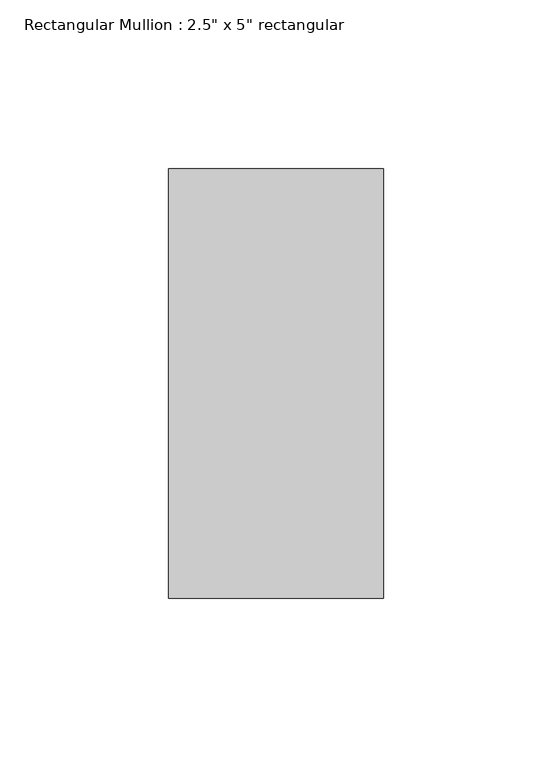
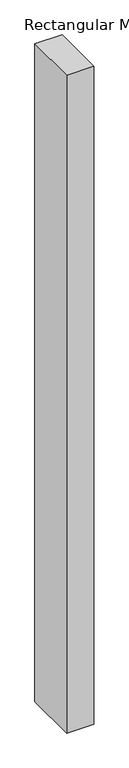
"""IFC4 building model written with IfcOpenShell, lengths in millimetres: member geometry."""

from ifc_helpers import new_model, si_unit, frame, origin, place, context, project, spatial, polyline, outline, extrude, source, transform, mapped, element, save


def member_4d9a94df(model_context):
    return source(origin(), model_context, "Body", "SweptSolid", [
        extrude(outline(polyline([(0.0, 63.5), (0.0, -63.5), (-63.5, -63.5), (-63.5, 63.5), (0.0, 63.5)])), frame((0.0, 0.0, -1611.7177577), z_axis=(0.0, 0.0, 1.0), x_axis=(1.0, 0.0, 0.0)), (0.0, 0.0, 1.0), 1611.7177577),
    ])


if __name__ == "__main__":
    model = new_model("IFC4")
    model_context = context("Model", 3, world=origin())
    ifc_project = project(units=[si_unit("LENGTHUNIT", "METRE", prefix="MILLI")], contexts=[model_context])
    site = spatial("IfcSite", under=ifc_project)
    building = spatial("IfcBuilding", under=site)
    placement = place(None, origin())
    member_shape = member_4d9a94df(model_context)
    element("IfcMember", 1, ObjectType="Rectangular Mullion : 2.5\" x 5\" rectangular", at=placement, inside=building, context=model_context, shape_type="MappedRepresentation", body=[
        mapped(member_shape, transform((0.0, 0.0, 0.0), x_axis=(1.0, 0.0, 0.0), y_axis=(0.0, 1.0, 0.0), z_axis=(0.0, 0.0, 1.0))),
    ])
    save(model, "model.ifc")

# Revit data of these elements
# Type "Rectangular Mullion : 2.5\" x 5\" rectangular"
#   built-in parameter 1007304 = 0.416667 (stored number, unit not read)
#   built-in parameter 1007301 = 0.104167 (stored number, unit not read)
#   built-in parameter 1007300 = 0.104167 (stored number, unit not read)
# Element 1 (IfcMember, "Rectangular Mullion : 2.5\" x 5\" rectangular")
#   Materials on its faces: "Aluminum"
# Materials
#   "Aluminum": class "Metal", colour RGB 247 247 247, transparency 0, Description = "Aluminum 6061", Cost = 0
